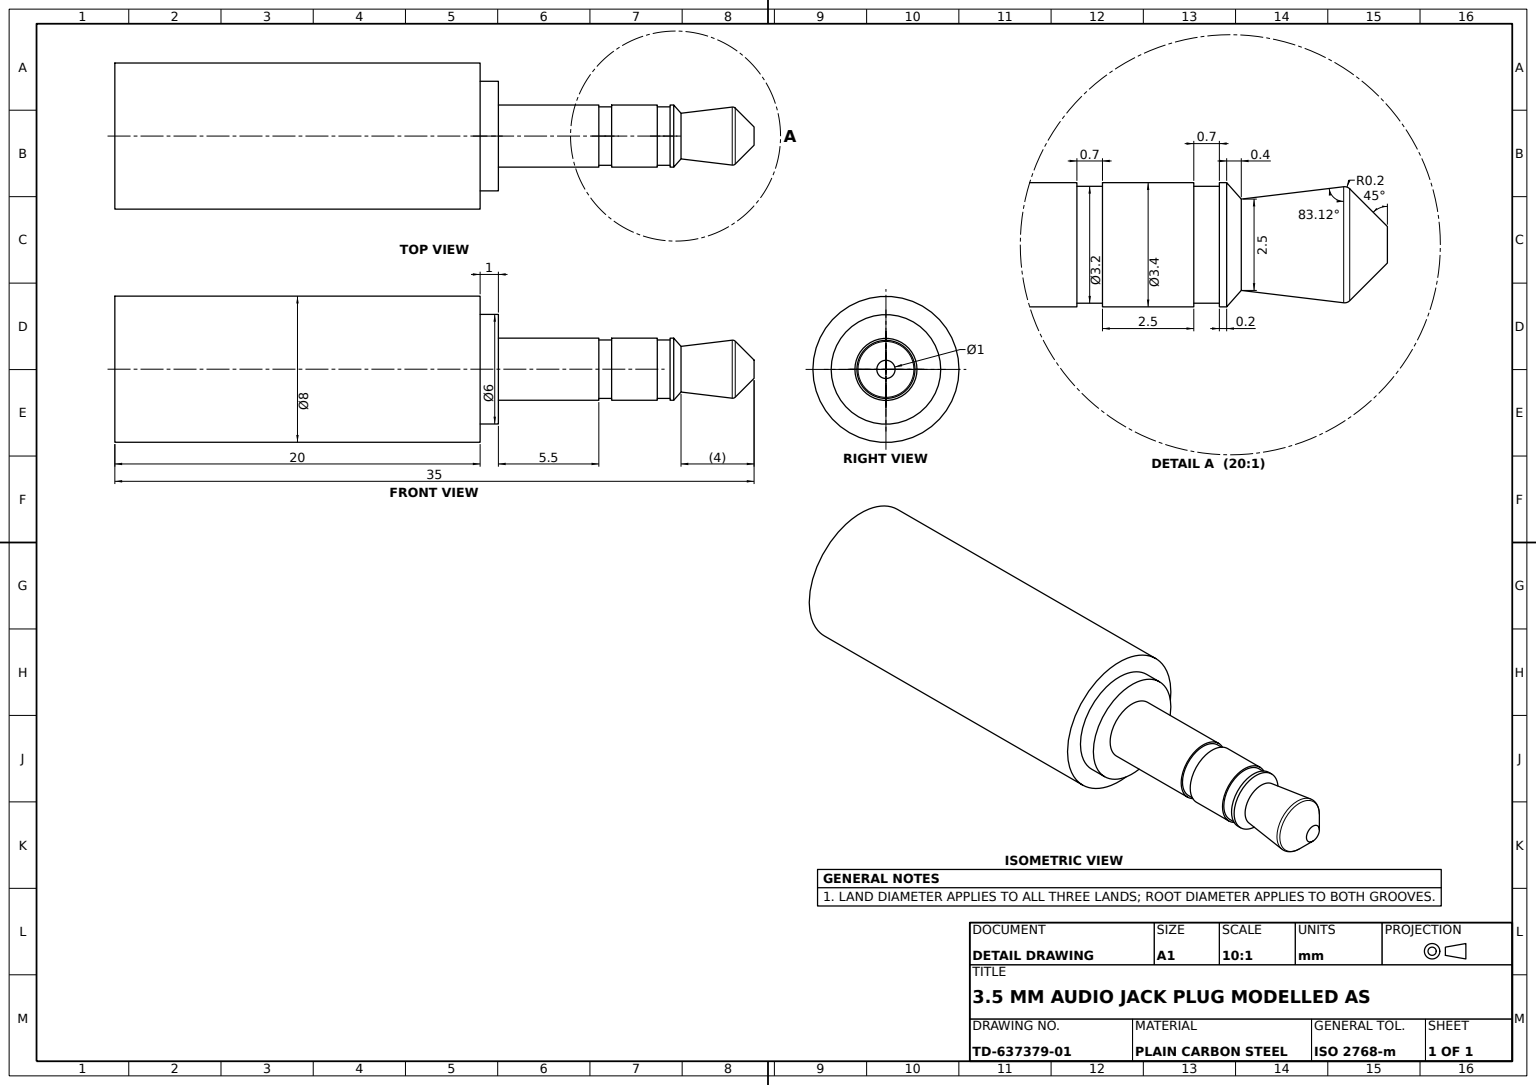
from build123d import *

# Parameters (mm, degrees)
EDGE_FILLET_R0_2_R = 0.2


with BuildPart() as part:
    # Plug Profile Sketch → Plug Body Revolve (revolve)
    with BuildSketch(Plane.XY, mode=Mode.PRIVATE) as plug_body_revolve_sk:
        Polygon((0, 0), (-35, 0), (-35, 4), (-15, 4), (-15, 3), (-14, 3), (-14, 1.7), (-8.5, 1.7), (-8.5, 1.6), (-7.8, 1.6), (-7.8, 1.7), (-5.3, 1.7), (-5.3, 1.6), (-4.6, 1.6), (-4.6, 1.7), (-4.4, 1.7), (-4, 1.25), (-1.1, 1.6), (0, 0.5), align=None)
    revolve(plug_body_revolve_sk.sketch.rotate(Axis((0, 0, 0), (-1, 0, 0)), 90), axis=Axis((0, 0, 0), (-1, 0, 0)))

    # Edge Fillet R0.2
    edge_fillet_r0_2_edges = [part.edges().sort_by_distance(p)[0] for p in [
        (-1.1, 0, 1.6),
    ]]
    fillet(edge_fillet_r0_2_edges, radius=EDGE_FILLET_R0_2_R)


solid = part.part
